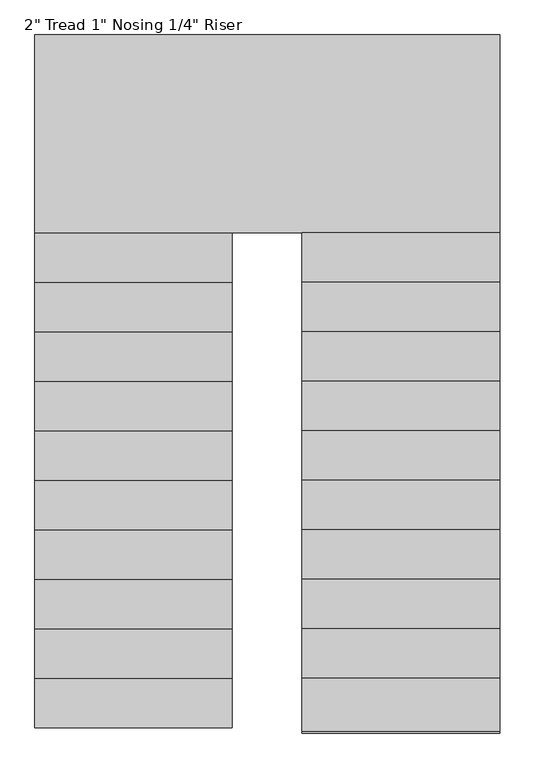
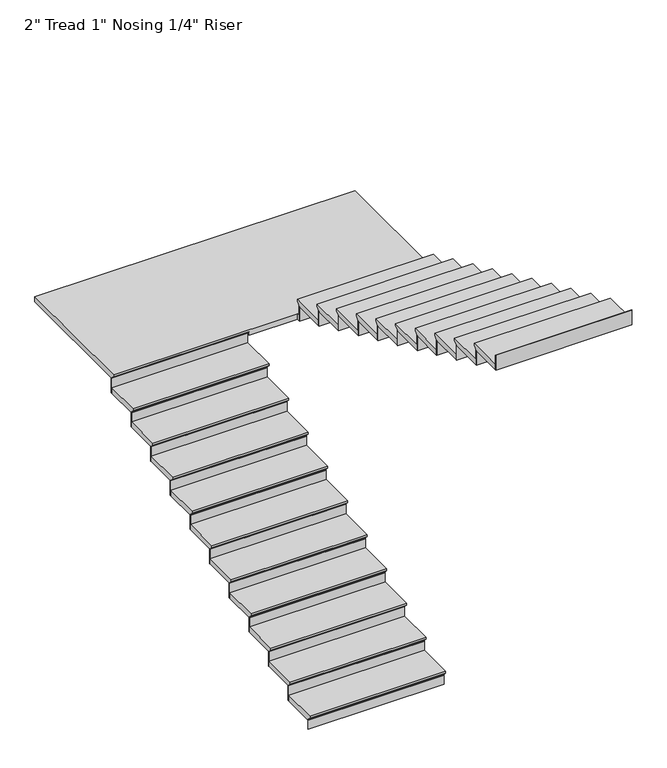
"""IFC4 building model written with IfcOpenShell, lengths in millimetres: stair flight geometry."""

from ifc_helpers import new_model, si_unit, origin, place, context, project, spatial, faceted_brep, source, transform, mapped, element, save


def stair_flight_185d1b01(model_context):
    return source(origin(), model_context, "Body", "Brep", [
        faceted_brep([(-629.5987998, 3364.6067329, 119.4954545), (-629.5987998, 3364.6067329, 138.5454545), (-1845.5417538, 3364.6067329, 138.5454545), (-1845.5417538, 3364.6067329, 119.4954545), (-629.5987998, 3390.0067329, 94.0954545), (-1845.5417538, 3390.0067329, 94.0954545), (-629.5987998, 3694.8067329, 138.5454545), (-1845.5417538, 3694.8067329, 138.5454545), (-1845.5417538, 3390.0067329, 87.7454545), (-1845.5417538, 3694.8067329, 87.7454545), (-629.5987998, 3694.8067329, 87.7454545), (-629.5987998, 3390.0067329, 87.7454545)], [[[0, 1, 2, 3]], [[4, 0, 3, 5]], [[2, 1, 6, 7]], [[8, 9, 10, 11]], [[2, 7, 9, 8, 5, 3]], [[8, 11, 4, 5]], [[6, 1, 0, 4, 11, 10]], [[7, 6, 10, 9]]]),
        faceted_brep([(-629.5987998, 3390.0067329, 87.7454545), (-629.5987998, 3390.0067329, 0.0), (-629.5987998, 3396.3567329, 0.0), (-629.5987998, 3396.3567329, 87.7454545), (-1845.5417538, 3390.0067329, 87.7454545), (-1845.5417538, 3396.3567329, 87.7454545), (-1845.5417538, 3396.3567329, 0.0), (-1845.5417538, 3390.0067329, 0.0)], [[[0, 1, 2, 3]], [[4, 5, 6, 7]], [[1, 0, 4, 7]], [[2, 1, 7, 6]], [[3, 2, 6, 5]], [[0, 3, 5, 4]]]),
        faceted_brep([(-629.5987998, 3694.8067329, 226.2909091), (-629.5987998, 3694.8067329, 87.7454545), (-629.5987998, 3701.1567329, 87.7454545), (-629.5987998, 3701.1567329, 226.2909091), (-1845.5417538, 3694.8067329, 226.2909091), (-1845.5417538, 3701.1567329, 226.2909091), (-1845.5417538, 3701.1567329, 87.7454545), (-1845.5417538, 3694.8067329, 87.7454545)], [[[0, 1, 2, 3]], [[4, 5, 6, 7]], [[1, 0, 4, 7]], [[2, 1, 7, 6]], [[3, 2, 6, 5]], [[0, 3, 5, 4]]]),
        faceted_brep([(-1845.5417538, 3669.4067329, 277.0909091), (-629.5987998, 3669.4067329, 277.0909091), (-629.5987998, 3999.6067329, 277.0909091), (-1845.5417538, 3999.6067329, 277.0909091), (-1845.5417538, 3694.8067329, 226.2909091), (-1845.5417538, 3999.6067329, 226.2909091), (-629.5987998, 3999.6067329, 226.2909091), (-629.5987998, 3694.8067329, 226.2909091), (-1845.5417538, 3694.8067329, 232.6409091), (-1845.5417538, 3669.4067329, 258.0409091), (-629.5987998, 3694.8067329, 232.6409091), (-629.5987998, 3669.4067329, 258.0409091)], [[[0, 1, 2, 3]], [[4, 5, 6, 7]], [[0, 3, 5, 4, 8, 9]], [[4, 7, 10, 8]], [[2, 1, 11, 10, 7, 6]], [[3, 2, 6, 5]], [[11, 1, 0, 9]], [[10, 11, 9, 8]]]),
        faceted_brep([(-629.5987998, 3999.6067329, 364.8363636), (-629.5987998, 3999.6067329, 226.2909091), (-629.5987998, 4005.9567329, 226.2909091), (-629.5987998, 4005.9567329, 364.8363636), (-1845.5417538, 3999.6067329, 364.8363636), (-1845.5417538, 4005.9567329, 364.8363636), (-1845.5417538, 4005.9567329, 226.2909091), (-1845.5417538, 3999.6067329, 226.2909091)], [[[0, 1, 2, 3]], [[4, 5, 6, 7]], [[1, 0, 4, 7]], [[2, 1, 7, 6]], [[3, 2, 6, 5]], [[0, 3, 5, 4]]]),
        faceted_brep([(-1845.5417538, 3974.2067329, 415.6363636), (-629.5987998, 3974.2067329, 415.6363636), (-629.5987998, 4304.4067329, 415.6363636), (-1845.5417538, 4304.4067329, 415.6363636), (-1845.5417538, 3999.6067329, 364.8363636), (-1845.5417538, 4304.4067329, 364.8363636), (-629.5987998, 4304.4067329, 364.8363636), (-629.5987998, 3999.6067329, 364.8363636), (-1845.5417538, 3999.6067329, 371.1863636), (-1845.5417538, 3974.2067329, 396.5863636), (-629.5987998, 3999.6067329, 371.1863636), (-629.5987998, 3974.2067329, 396.5863636)], [[[0, 1, 2, 3]], [[4, 5, 6, 7]], [[0, 3, 5, 4, 8, 9]], [[4, 7, 10, 8]], [[2, 1, 11, 10, 7, 6]], [[3, 2, 6, 5]], [[11, 1, 0, 9]], [[10, 11, 9, 8]]]),
        faceted_brep([(-629.5987998, 4304.4067329, 503.3818182), (-629.5987998, 4304.4067329, 364.8363636), (-629.5987998, 4310.7567329, 364.8363636), (-629.5987998, 4310.7567329, 503.3818182), (-1845.5417538, 4304.4067329, 503.3818182), (-1845.5417538, 4310.7567329, 503.3818182), (-1845.5417538, 4310.7567329, 364.8363636), (-1845.5417538, 4304.4067329, 364.8363636)], [[[0, 1, 2, 3]], [[4, 5, 6, 7]], [[1, 0, 4, 7]], [[2, 1, 7, 6]], [[3, 2, 6, 5]], [[0, 3, 5, 4]]]),
        faceted_brep([(-1845.5417538, 4279.0067329, 554.1818182), (-629.5987998, 4279.0067329, 554.1818182), (-629.5987998, 4609.2067329, 554.1818182), (-1845.5417538, 4609.2067329, 554.1818182), (-1845.5417538, 4304.4067329, 503.3818182), (-1845.5417538, 4609.2067329, 503.3818182), (-629.5987998, 4609.2067329, 503.3818182), (-629.5987998, 4304.4067329, 503.3818182), (-1845.5417538, 4304.4067329, 509.7318182), (-1845.5417538, 4279.0067329, 535.1318182), (-629.5987998, 4304.4067329, 509.7318182), (-629.5987998, 4279.0067329, 535.1318182)], [[[0, 1, 2, 3]], [[4, 5, 6, 7]], [[0, 3, 5, 4, 8, 9]], [[4, 7, 10, 8]], [[2, 1, 11, 10, 7, 6]], [[3, 2, 6, 5]], [[11, 1, 0, 9]], [[10, 11, 9, 8]]]),
        faceted_brep([(-629.5987998, 4609.2067329, 641.9272727), (-629.5987998, 4609.2067329, 503.3818182), (-629.5987998, 4615.5567329, 503.3818182), (-629.5987998, 4615.5567329, 641.9272727), (-1845.5417538, 4609.2067329, 641.9272727), (-1845.5417538, 4615.5567329, 641.9272727), (-1845.5417538, 4615.5567329, 503.3818182), (-1845.5417538, 4609.2067329, 503.3818182)], [[[0, 1, 2, 3]], [[4, 5, 6, 7]], [[1, 0, 4, 7]], [[2, 1, 7, 6]], [[3, 2, 6, 5]], [[0, 3, 5, 4]]]),
        faceted_brep([(-1845.5417538, 4583.8067329, 692.7272727), (-629.5987998, 4583.8067329, 692.7272727), (-629.5987998, 4914.0067329, 692.7272727), (-1845.5417538, 4914.0067329, 692.7272727), (-1845.5417538, 4609.2067329, 641.9272727), (-1845.5417538, 4914.0067329, 641.9272727), (-629.5987998, 4914.0067329, 641.9272727), (-629.5987998, 4609.2067329, 641.9272727), (-1845.5417538, 4609.2067329, 648.2772727), (-1845.5417538, 4583.8067329, 673.6772727), (-629.5987998, 4609.2067329, 648.2772727), (-629.5987998, 4583.8067329, 673.6772727)], [[[0, 1, 2, 3]], [[4, 5, 6, 7]], [[0, 3, 5, 4, 8, 9]], [[4, 7, 10, 8]], [[2, 1, 11, 10, 7, 6]], [[3, 2, 6, 5]], [[11, 1, 0, 9]], [[10, 11, 9, 8]]]),
        faceted_brep([(-629.5987998, 4914.0067329, 780.4727273), (-629.5987998, 4914.0067329, 641.9272727), (-629.5987998, 4920.3567329, 641.9272727), (-629.5987998, 4920.3567329, 780.4727273), (-1845.5417538, 4914.0067329, 780.4727273), (-1845.5417538, 4920.3567329, 780.4727273), (-1845.5417538, 4920.3567329, 641.9272727), (-1845.5417538, 4914.0067329, 641.9272727)], [[[0, 1, 2, 3]], [[4, 5, 6, 7]], [[1, 0, 4, 7]], [[2, 1, 7, 6]], [[3, 2, 6, 5]], [[0, 3, 5, 4]]]),
        faceted_brep([(-1845.5417538, 4888.6067329, 831.2727273), (-629.5987998, 4888.6067329, 831.2727273), (-629.5987998, 5218.8067329, 831.2727273), (-1845.5417538, 5218.8067329, 831.2727273), (-1845.5417538, 4914.0067329, 780.4727273), (-1845.5417538, 5218.8067329, 780.4727273), (-629.5987998, 5218.8067329, 780.4727273), (-629.5987998, 4914.0067329, 780.4727273), (-1845.5417538, 4914.0067329, 786.8227273), (-1845.5417538, 4888.6067329, 812.2227273), (-629.5987998, 4914.0067329, 786.8227273), (-629.5987998, 4888.6067329, 812.2227273)], [[[0, 1, 2, 3]], [[4, 5, 6, 7]], [[0, 3, 5, 4, 8, 9]], [[4, 7, 10, 8]], [[2, 1, 11, 10, 7, 6]], [[3, 2, 6, 5]], [[11, 1, 0, 9]], [[10, 11, 9, 8]]]),
        faceted_brep([(-629.5987998, 5218.8067329, 919.0181818), (-629.5987998, 5218.8067329, 780.4727273), (-629.5987998, 5225.1567329, 780.4727273), (-629.5987998, 5225.1567329, 919.0181818), (-1845.5417538, 5218.8067329, 919.0181818), (-1845.5417538, 5225.1567329, 919.0181818), (-1845.5417538, 5225.1567329, 780.4727273), (-1845.5417538, 5218.8067329, 780.4727273)], [[[0, 1, 2, 3]], [[4, 5, 6, 7]], [[1, 0, 4, 7]], [[2, 1, 7, 6]], [[3, 2, 6, 5]], [[0, 3, 5, 4]]]),
        faceted_brep([(-1845.5417538, 5193.4067329, 969.8181818), (-629.5987998, 5193.4067329, 969.8181818), (-629.5987998, 5523.6067329, 969.8181818), (-1845.5417538, 5523.6067329, 969.8181818), (-1845.5417538, 5218.8067329, 919.0181818), (-1845.5417538, 5523.6067329, 919.0181818), (-629.5987998, 5523.6067329, 919.0181818), (-629.5987998, 5218.8067329, 919.0181818), (-1845.5417538, 5218.8067329, 925.3681818), (-1845.5417538, 5193.4067329, 950.7681818), (-629.5987998, 5218.8067329, 925.3681818), (-629.5987998, 5193.4067329, 950.7681818)], [[[0, 1, 2, 3]], [[4, 5, 6, 7]], [[0, 3, 5, 4, 8, 9]], [[4, 7, 10, 8]], [[2, 1, 11, 10, 7, 6]], [[3, 2, 6, 5]], [[11, 1, 0, 9]], [[10, 11, 9, 8]]]),
        faceted_brep([(-629.5987998, 5523.6067329, 1057.5636364), (-629.5987998, 5523.6067329, 919.0181818), (-629.5987998, 5529.9567329, 919.0181818), (-629.5987998, 5529.9567329, 1057.5636364), (-1845.5417538, 5523.6067329, 1057.5636364), (-1845.5417538, 5529.9567329, 1057.5636364), (-1845.5417538, 5529.9567329, 919.0181818), (-1845.5417538, 5523.6067329, 919.0181818)], [[[0, 1, 2, 3]], [[4, 5, 6, 7]], [[1, 0, 4, 7]], [[2, 1, 7, 6]], [[3, 2, 6, 5]], [[0, 3, 5, 4]]]),
        faceted_brep([(-1845.5417538, 5498.2067329, 1108.3636364), (-629.5987998, 5498.2067329, 1108.3636364), (-629.5987998, 5828.4067329, 1108.3636364), (-1845.5417538, 5828.4067329, 1108.3636364), (-1845.5417538, 5523.6067329, 1057.5636364), (-1845.5417538, 5828.4067329, 1057.5636364), (-629.5987998, 5828.4067329, 1057.5636364), (-629.5987998, 5523.6067329, 1057.5636364), (-1845.5417538, 5523.6067329, 1063.9136364), (-1845.5417538, 5498.2067329, 1089.3136364), (-629.5987998, 5523.6067329, 1063.9136364), (-629.5987998, 5498.2067329, 1089.3136364)], [[[0, 1, 2, 3]], [[4, 5, 6, 7]], [[0, 3, 5, 4, 8, 9]], [[4, 7, 10, 8]], [[2, 1, 11, 10, 7, 6]], [[3, 2, 6, 5]], [[11, 1, 0, 9]], [[10, 11, 9, 8]]]),
        faceted_brep([(-629.5987998, 5828.4067329, 1196.1090909), (-629.5987998, 5828.4067329, 1057.5636364), (-629.5987998, 5834.7567329, 1057.5636364), (-629.5987998, 5834.7567329, 1196.1090909), (-1845.5417538, 5828.4067329, 1196.1090909), (-1845.5417538, 5834.7567329, 1196.1090909), (-1845.5417538, 5834.7567329, 1057.5636364), (-1845.5417538, 5828.4067329, 1057.5636364)], [[[0, 1, 2, 3]], [[4, 5, 6, 7]], [[1, 0, 4, 7]], [[2, 1, 7, 6]], [[3, 2, 6, 5]], [[0, 3, 5, 4]]]),
        faceted_brep([(-1845.5417538, 5803.0067329, 1246.9090909), (-629.5987998, 5803.0067329, 1246.9090909), (-629.5987998, 6133.2067329, 1246.9090909), (-1845.5417538, 6133.2067329, 1246.9090909), (-1845.5417538, 5828.4067329, 1196.1090909), (-1845.5417538, 6133.2067329, 1196.1090909), (-629.5987998, 6133.2067329, 1196.1090909), (-629.5987998, 5828.4067329, 1196.1090909), (-1845.5417538, 5828.4067329, 1202.4590909), (-1845.5417538, 5803.0067329, 1227.8590909), (-629.5987998, 5828.4067329, 1202.4590909), (-629.5987998, 5803.0067329, 1227.8590909)], [[[0, 1, 2, 3]], [[4, 5, 6, 7]], [[0, 3, 5, 4, 8, 9]], [[4, 7, 10, 8]], [[2, 1, 11, 10, 7, 6]], [[3, 2, 6, 5]], [[11, 1, 0, 9]], [[10, 11, 9, 8]]]),
        faceted_brep([(-629.5987998, 6133.2067329, 1334.6545455), (-629.5987998, 6133.2067329, 1196.1090909), (-629.5987998, 6139.5567329, 1196.1090909), (-629.5987998, 6139.5567329, 1334.6545455), (-1845.5417538, 6133.2067329, 1334.6545455), (-1845.5417538, 6139.5567329, 1334.6545455), (-1845.5417538, 6139.5567329, 1196.1090909), (-1845.5417538, 6133.2067329, 1196.1090909)], [[[0, 1, 2, 3]], [[4, 5, 6, 7]], [[1, 0, 4, 7]], [[2, 1, 7, 6]], [[3, 2, 6, 5]], [[0, 3, 5, 4]]]),
        faceted_brep([(-1845.5417538, 6107.8067329, 1385.4545455), (-629.5987998, 6107.8067329, 1385.4545455), (-629.5987998, 6438.0067329, 1385.4545455), (-1845.5417538, 6438.0067329, 1385.4545455), (-1845.5417538, 6133.2067329, 1334.6545455), (-1845.5417538, 6438.0067329, 1334.6545455), (-629.5987998, 6438.0067329, 1334.6545455), (-629.5987998, 6133.2067329, 1334.6545455), (-1845.5417538, 6133.2067329, 1341.0045455), (-1845.5417538, 6107.8067329, 1366.4045455), (-629.5987998, 6133.2067329, 1341.0045455), (-629.5987998, 6107.8067329, 1366.4045455)], [[[0, 1, 2, 3]], [[4, 5, 6, 7]], [[0, 3, 5, 4, 8, 9]], [[4, 7, 10, 8]], [[2, 1, 11, 10, 7, 6]], [[3, 2, 6, 5]], [[11, 1, 0, 9]], [[10, 11, 9, 8]]]),
        faceted_brep([(-629.5987998, 6438.0067329, 1473.2), (-629.5987998, 6438.0067329, 1334.6545455), (-629.5987998, 6444.3567329, 1334.6545455), (-629.5987998, 6444.3567329, 1473.2), (-1845.5417538, 6438.0067329, 1473.2), (-1845.5417538, 6444.3567329, 1473.2), (-1845.5417538, 6444.3567329, 1334.6545455), (-1845.5417538, 6438.0067329, 1334.6545455)], [[[0, 1, 2, 3]], [[4, 5, 6, 7]], [[1, 0, 4, 7]], [[2, 1, 7, 6]], [[3, 2, 6, 5]], [[0, 3, 5, 4]]]),
        faceted_brep([(1021.4012085, 6387.2067329, 1524.0), (1021.4012085, 7631.8067329, 1524.0), (-1845.5417538, 7631.8067329, 1524.0), (-1845.5417538, 6412.6067329, 1524.0), (-197.7987915, 6412.6067329, 1524.0), (-197.7987915, 6387.2067329, 1524.0), (1021.4012085, 7631.8067329, 1473.2), (1021.4012085, 6387.2067329, 1473.2), (-197.7987915, 6387.2067329, 1473.2), (-197.7987915, 6412.6067329, 1473.2), (-629.5987998, 6412.6067329, 1473.2), (-629.5987998, 6438.0067329, 1473.2), (-1845.5417538, 6438.0067329, 1473.2), (-1845.5417538, 7631.8067329, 1473.2), (-629.5987998, 6438.0067329, 1479.55), (-1845.5417538, 6438.0067329, 1479.55), (-1845.5417538, 6412.6067329, 1504.95), (-629.5987998, 6412.6067329, 1504.95)], [[[0, 1, 2, 3, 4, 5]], [[6, 7, 8, 9, 10, 11, 12, 13]], [[1, 0, 7, 6]], [[2, 1, 6, 13]], [[12, 11, 14, 15]], [[4, 3, 16, 17, 10, 9]], [[5, 4, 9, 8]], [[0, 5, 8, 7]], [[16, 15, 14, 17]], [[3, 2, 13, 12, 15, 16]], [[11, 10, 17, 14]]]),
        faceted_brep([(-197.7987915, 6387.2067329, 1611.7454545), (-197.7987915, 6387.2067329, 1473.2), (-197.7987915, 6380.8567329, 1473.2), (-197.7987915, 6380.8567329, 1611.7454545), (1021.4012085, 6387.2067329, 1611.7454545), (1021.4012085, 6380.8567329, 1611.7454545), (1021.4012085, 6380.8567329, 1473.2), (1021.4012085, 6387.2067329, 1473.2)], [[[0, 1, 2, 3]], [[4, 5, 6, 7]], [[1, 0, 4, 7]], [[2, 1, 7, 6]], [[3, 2, 6, 5]], [[0, 3, 5, 4]]]),
        faceted_brep([(1021.4012085, 6412.6067329, 1662.5454545), (-197.7987915, 6412.6067329, 1662.5454545), (-197.7987915, 6082.4067329, 1662.5454545), (1021.4012085, 6082.4067329, 1662.5454545), (1021.4012085, 6387.2067329, 1611.7454545), (1021.4012085, 6082.4067329, 1611.7454545), (-197.7987915, 6082.4067329, 1611.7454545), (-197.7987915, 6387.2067329, 1611.7454545), (1021.4012085, 6387.2067329, 1618.0954545), (1021.4012085, 6412.6067329, 1643.4954545), (-197.7987915, 6387.2067329, 1618.0954545), (-197.7987915, 6412.6067329, 1643.4954545)], [[[0, 1, 2, 3]], [[4, 5, 6, 7]], [[0, 3, 5, 4, 8, 9]], [[4, 7, 10, 8]], [[2, 1, 11, 10, 7, 6]], [[3, 2, 6, 5]], [[11, 1, 0, 9]], [[10, 11, 9, 8]]]),
        faceted_brep([(-197.7987915, 6082.4067329, 1750.2909091), (-197.7987915, 6082.4067329, 1611.7454545), (-197.7987915, 6076.0567329, 1611.7454545), (-197.7987915, 6076.0567329, 1750.2909091), (1021.4012085, 6082.4067329, 1750.2909091), (1021.4012085, 6076.0567329, 1750.2909091), (1021.4012085, 6076.0567329, 1611.7454545), (1021.4012085, 6082.4067329, 1611.7454545)], [[[0, 1, 2, 3]], [[4, 5, 6, 7]], [[1, 0, 4, 7]], [[2, 1, 7, 6]], [[3, 2, 6, 5]], [[0, 3, 5, 4]]]),
        faceted_brep([(1021.4012085, 6107.8067329, 1801.0909091), (-197.7987915, 6107.8067329, 1801.0909091), (-197.7987915, 5777.6067329, 1801.0909091), (1021.4012085, 5777.6067329, 1801.0909091), (1021.4012085, 6082.4067329, 1750.2909091), (1021.4012085, 5777.6067329, 1750.2909091), (-197.7987915, 5777.6067329, 1750.2909091), (-197.7987915, 6082.4067329, 1750.2909091), (1021.4012085, 6082.4067329, 1756.6409091), (1021.4012085, 6107.8067329, 1782.0409091), (-197.7987915, 6082.4067329, 1756.6409091), (-197.7987915, 6107.8067329, 1782.0409091)], [[[0, 1, 2, 3]], [[4, 5, 6, 7]], [[0, 3, 5, 4, 8, 9]], [[4, 7, 10, 8]], [[2, 1, 11, 10, 7, 6]], [[3, 2, 6, 5]], [[11, 1, 0, 9]], [[10, 11, 9, 8]]]),
        faceted_brep([(-197.7987915, 5777.6067329, 1888.8363636), (-197.7987915, 5777.6067329, 1750.2909091), (-197.7987915, 5771.2567329, 1750.2909091), (-197.7987915, 5771.2567329, 1888.8363636), (1021.4012085, 5777.6067329, 1888.8363636), (1021.4012085, 5771.2567329, 1888.8363636), (1021.4012085, 5771.2567329, 1750.2909091), (1021.4012085, 5777.6067329, 1750.2909091)], [[[0, 1, 2, 3]], [[4, 5, 6, 7]], [[1, 0, 4, 7]], [[2, 1, 7, 6]], [[3, 2, 6, 5]], [[0, 3, 5, 4]]]),
        faceted_brep([(1021.4012085, 5803.0067329, 1939.6363636), (-197.7987915, 5803.0067329, 1939.6363636), (-197.7987915, 5472.8067329, 1939.6363636), (1021.4012085, 5472.8067329, 1939.6363636), (1021.4012085, 5777.6067329, 1888.8363636), (1021.4012085, 5472.8067329, 1888.8363636), (-197.7987915, 5472.8067329, 1888.8363636), (-197.7987915, 5777.6067329, 1888.8363636), (1021.4012085, 5777.6067329, 1895.1863636), (1021.4012085, 5803.0067329, 1920.5863636), (-197.7987915, 5777.6067329, 1895.1863636), (-197.7987915, 5803.0067329, 1920.5863636)], [[[0, 1, 2, 3]], [[4, 5, 6, 7]], [[0, 3, 5, 4, 8, 9]], [[4, 7, 10, 8]], [[2, 1, 11, 10, 7, 6]], [[3, 2, 6, 5]], [[11, 1, 0, 9]], [[10, 11, 9, 8]]]),
        faceted_brep([(-197.7987915, 5472.8067329, 2027.3818182), (-197.7987915, 5472.8067329, 1888.8363636), (-197.7987915, 5466.4567329, 1888.8363636), (-197.7987915, 5466.4567329, 2027.3818182), (1021.4012085, 5472.8067329, 2027.3818182), (1021.4012085, 5466.4567329, 2027.3818182), (1021.4012085, 5466.4567329, 1888.8363636), (1021.4012085, 5472.8067329, 1888.8363636)], [[[0, 1, 2, 3]], [[4, 5, 6, 7]], [[1, 0, 4, 7]], [[2, 1, 7, 6]], [[3, 2, 6, 5]], [[0, 3, 5, 4]]]),
        faceted_brep([(1021.4012085, 5498.2067329, 2078.1818182), (-197.7987915, 5498.2067329, 2078.1818182), (-197.7987915, 5168.0067329, 2078.1818182), (1021.4012085, 5168.0067329, 2078.1818182), (1021.4012085, 5472.8067329, 2027.3818182), (1021.4012085, 5168.0067329, 2027.3818182), (-197.7987915, 5168.0067329, 2027.3818182), (-197.7987915, 5472.8067329, 2027.3818182), (1021.4012085, 5472.8067329, 2033.7318182), (1021.4012085, 5498.2067329, 2059.1318182), (-197.7987915, 5472.8067329, 2033.7318182), (-197.7987915, 5498.2067329, 2059.1318182)], [[[0, 1, 2, 3]], [[4, 5, 6, 7]], [[0, 3, 5, 4, 8, 9]], [[4, 7, 10, 8]], [[2, 1, 11, 10, 7, 6]], [[3, 2, 6, 5]], [[11, 1, 0, 9]], [[10, 11, 9, 8]]]),
        faceted_brep([(-197.7987915, 5168.0067329, 2165.9272727), (-197.7987915, 5168.0067329, 2027.3818182), (-197.7987915, 5161.6567329, 2027.3818182), (-197.7987915, 5161.6567329, 2165.9272727), (1021.4012085, 5168.0067329, 2165.9272727), (1021.4012085, 5161.6567329, 2165.9272727), (1021.4012085, 5161.6567329, 2027.3818182), (1021.4012085, 5168.0067329, 2027.3818182)], [[[0, 1, 2, 3]], [[4, 5, 6, 7]], [[1, 0, 4, 7]], [[2, 1, 7, 6]], [[3, 2, 6, 5]], [[0, 3, 5, 4]]]),
        faceted_brep([(1021.4012085, 5193.4067329, 2216.7272727), (-197.7987915, 5193.4067329, 2216.7272727), (-197.7987915, 4863.2067329, 2216.7272727), (1021.4012085, 4863.2067329, 2216.7272727), (1021.4012085, 5168.0067329, 2165.9272727), (1021.4012085, 4863.2067329, 2165.9272727), (-197.7987915, 4863.2067329, 2165.9272727), (-197.7987915, 5168.0067329, 2165.9272727), (1021.4012085, 5168.0067329, 2172.2772727), (1021.4012085, 5193.4067329, 2197.6772727), (-197.7987915, 5168.0067329, 2172.2772727), (-197.7987915, 5193.4067329, 2197.6772727)], [[[0, 1, 2, 3]], [[4, 5, 6, 7]], [[0, 3, 5, 4, 8, 9]], [[4, 7, 10, 8]], [[2, 1, 11, 10, 7, 6]], [[3, 2, 6, 5]], [[11, 1, 0, 9]], [[10, 11, 9, 8]]]),
        faceted_brep([(-197.7987915, 4863.2067329, 2304.4727273), (-197.7987915, 4863.2067329, 2165.9272727), (-197.7987915, 4856.8567329, 2165.9272727), (-197.7987915, 4856.8567329, 2304.4727273), (1021.4012085, 4863.2067329, 2304.4727273), (1021.4012085, 4856.8567329, 2304.4727273), (1021.4012085, 4856.8567329, 2165.9272727), (1021.4012085, 4863.2067329, 2165.9272727)], [[[0, 1, 2, 3]], [[4, 5, 6, 7]], [[1, 0, 4, 7]], [[2, 1, 7, 6]], [[3, 2, 6, 5]], [[0, 3, 5, 4]]]),
        faceted_brep([(1021.4012085, 4888.6067329, 2355.2727273), (-197.7987915, 4888.6067329, 2355.2727273), (-197.7987915, 4558.4067329, 2355.2727273), (1021.4012085, 4558.4067329, 2355.2727273), (1021.4012085, 4863.2067329, 2304.4727273), (1021.4012085, 4558.4067329, 2304.4727273), (-197.7987915, 4558.4067329, 2304.4727273), (-197.7987915, 4863.2067329, 2304.4727273), (1021.4012085, 4863.2067329, 2310.8227273), (1021.4012085, 4888.6067329, 2336.2227273), (-197.7987915, 4863.2067329, 2310.8227273), (-197.7987915, 4888.6067329, 2336.2227273)], [[[0, 1, 2, 3]], [[4, 5, 6, 7]], [[0, 3, 5, 4, 8, 9]], [[4, 7, 10, 8]], [[2, 1, 11, 10, 7, 6]], [[3, 2, 6, 5]], [[11, 1, 0, 9]], [[10, 11, 9, 8]]]),
        faceted_brep([(-197.7987915, 4558.4067329, 2443.0181818), (-197.7987915, 4558.4067329, 2304.4727273), (-197.7987915, 4552.0567329, 2304.4727273), (-197.7987915, 4552.0567329, 2443.0181818), (1021.4012085, 4558.4067329, 2443.0181818), (1021.4012085, 4552.0567329, 2443.0181818), (1021.4012085, 4552.0567329, 2304.4727273), (1021.4012085, 4558.4067329, 2304.4727273)], [[[0, 1, 2, 3]], [[4, 5, 6, 7]], [[1, 0, 4, 7]], [[2, 1, 7, 6]], [[3, 2, 6, 5]], [[0, 3, 5, 4]]]),
        faceted_brep([(1021.4012085, 4583.8067329, 2493.8181818), (-197.7987915, 4583.8067329, 2493.8181818), (-197.7987915, 4253.6067329, 2493.8181818), (1021.4012085, 4253.6067329, 2493.8181818), (1021.4012085, 4558.4067329, 2443.0181818), (1021.4012085, 4253.6067329, 2443.0181818), (-197.7987915, 4253.6067329, 2443.0181818), (-197.7987915, 4558.4067329, 2443.0181818), (1021.4012085, 4558.4067329, 2449.3681818), (1021.4012085, 4583.8067329, 2474.7681818), (-197.7987915, 4558.4067329, 2449.3681818), (-197.7987915, 4583.8067329, 2474.7681818)], [[[0, 1, 2, 3]], [[4, 5, 6, 7]], [[0, 3, 5, 4, 8, 9]], [[4, 7, 10, 8]], [[2, 1, 11, 10, 7, 6]], [[3, 2, 6, 5]], [[11, 1, 0, 9]], [[10, 11, 9, 8]]]),
        faceted_brep([(-197.7987915, 4253.6067329, 2581.5636364), (-197.7987915, 4253.6067329, 2443.0181818), (-197.7987915, 4247.2567329, 2443.0181818), (-197.7987915, 4247.2567329, 2581.5636364), (1021.4012085, 4253.6067329, 2581.5636364), (1021.4012085, 4247.2567329, 2581.5636364), (1021.4012085, 4247.2567329, 2443.0181818), (1021.4012085, 4253.6067329, 2443.0181818)], [[[0, 1, 2, 3]], [[4, 5, 6, 7]], [[1, 0, 4, 7]], [[2, 1, 7, 6]], [[3, 2, 6, 5]], [[0, 3, 5, 4]]]),
        faceted_brep([(1021.4012085, 4279.0067329, 2632.3636364), (-197.7987915, 4279.0067329, 2632.3636364), (-197.7987915, 3948.8067329, 2632.3636364), (1021.4012085, 3948.8067329, 2632.3636364), (1021.4012085, 4253.6067329, 2581.5636364), (1021.4012085, 3948.8067329, 2581.5636364), (-197.7987915, 3948.8067329, 2581.5636364), (-197.7987915, 4253.6067329, 2581.5636364), (1021.4012085, 4253.6067329, 2587.9136364), (1021.4012085, 4279.0067329, 2613.3136364), (-197.7987915, 4253.6067329, 2587.9136364), (-197.7987915, 4279.0067329, 2613.3136364)], [[[0, 1, 2, 3]], [[4, 5, 6, 7]], [[0, 3, 5, 4, 8, 9]], [[4, 7, 10, 8]], [[2, 1, 11, 10, 7, 6]], [[3, 2, 6, 5]], [[11, 1, 0, 9]], [[10, 11, 9, 8]]]),
        faceted_brep([(-197.7987915, 3948.8067329, 2720.1090909), (-197.7987915, 3948.8067329, 2581.5636364), (-197.7987915, 3942.4567329, 2581.5636364), (-197.7987915, 3942.4567329, 2720.1090909), (1021.4012085, 3948.8067329, 2720.1090909), (1021.4012085, 3942.4567329, 2720.1090909), (1021.4012085, 3942.4567329, 2581.5636364), (1021.4012085, 3948.8067329, 2581.5636364)], [[[0, 1, 2, 3]], [[4, 5, 6, 7]], [[1, 0, 4, 7]], [[2, 1, 7, 6]], [[3, 2, 6, 5]], [[0, 3, 5, 4]]]),
        faceted_brep([(1021.4012085, 3974.2067329, 2770.9090909), (-197.7987915, 3974.2067329, 2770.9090909), (-197.7987915, 3644.0067329, 2770.9090909), (1021.4012085, 3644.0067329, 2770.9090909), (1021.4012085, 3948.8067329, 2720.1090909), (1021.4012085, 3644.0067329, 2720.1090909), (-197.7987915, 3644.0067329, 2720.1090909), (-197.7987915, 3948.8067329, 2720.1090909), (1021.4012085, 3948.8067329, 2726.4590909), (1021.4012085, 3974.2067329, 2751.8590909), (-197.7987915, 3948.8067329, 2726.4590909), (-197.7987915, 3974.2067329, 2751.8590909)], [[[0, 1, 2, 3]], [[4, 5, 6, 7]], [[0, 3, 5, 4, 8, 9]], [[4, 7, 10, 8]], [[2, 1, 11, 10, 7, 6]], [[3, 2, 6, 5]], [[11, 1, 0, 9]], [[10, 11, 9, 8]]]),
        faceted_brep([(-197.7987915, 3644.0067329, 2858.6545455), (-197.7987915, 3644.0067329, 2720.1090909), (-197.7987915, 3637.6567329, 2720.1090909), (-197.7987915, 3637.6567329, 2858.6545455), (1021.4012085, 3644.0067329, 2858.6545455), (1021.4012085, 3637.6567329, 2858.6545455), (1021.4012085, 3637.6567329, 2720.1090909), (1021.4012085, 3644.0067329, 2720.1090909)], [[[0, 1, 2, 3]], [[4, 5, 6, 7]], [[1, 0, 4, 7]], [[2, 1, 7, 6]], [[3, 2, 6, 5]], [[0, 3, 5, 4]]]),
        faceted_brep([(-197.7987915, 3339.2067329, 2997.2), (-197.7987915, 3339.2067329, 2858.6545455), (-197.7987915, 3332.8567329, 2858.6545455), (-197.7987915, 3332.8567329, 2997.2), (1021.4012085, 3339.2067329, 2997.2), (1021.4012085, 3332.8567329, 2997.2), (1021.4012085, 3332.8567329, 2858.6545455), (1021.4012085, 3339.2067329, 2858.6545455)], [[[0, 1, 2, 3]], [[4, 5, 6, 7]], [[1, 0, 4, 7]], [[2, 1, 7, 6]], [[3, 2, 6, 5]], [[0, 3, 5, 4]]]),
        faceted_brep([(1021.4012085, 3669.4067329, 2909.4545455), (-197.7987915, 3669.4067329, 2909.4545455), (-197.7987915, 3339.2067329, 2909.4545455), (1021.4012085, 3339.2067329, 2909.4545455), (1021.4012085, 3644.0067329, 2858.6545455), (1021.4012085, 3339.2067329, 2858.6545455), (-197.7987915, 3339.2067329, 2858.6545455), (-197.7987915, 3644.0067329, 2858.6545455), (1021.4012085, 3644.0067329, 2865.0045455), (1021.4012085, 3669.4067329, 2890.4045455), (-197.7987915, 3644.0067329, 2865.0045455), (-197.7987915, 3669.4067329, 2890.4045455)], [[[0, 1, 2, 3]], [[4, 5, 6, 7]], [[0, 3, 5, 4, 8, 9]], [[4, 7, 10, 8]], [[2, 1, 11, 10, 7, 6]], [[3, 2, 6, 5]], [[11, 1, 0, 9]], [[10, 11, 9, 8]]]),
    ])


if __name__ == "__main__":
    model = new_model("IFC4")
    model_context = context("Model", 3, world=origin())
    ifc_project = project(units=[si_unit("LENGTHUNIT", "METRE", prefix="MILLI")], contexts=[model_context])
    site = spatial("IfcSite", under=ifc_project)
    building = spatial("IfcBuilding", under=site)
    placement = place(None, origin())
    stair_flight_shape = stair_flight_185d1b01(model_context)
    element("IfcStairFlight", 1, ObjectType="2\" Tread 1\" Nosing 1/4\" Riser", at=placement, inside=building, context=model_context, shape_type="MappedRepresentation", body=[
        mapped(stair_flight_shape, transform((0.0, 0.0, 0.0), x_axis=(1.0, 0.0, 0.0), y_axis=(0.0, 1.0, 0.0), z_axis=(0.0, 0.0, 1.0))),
    ])
    save(model, "model.ifc")
